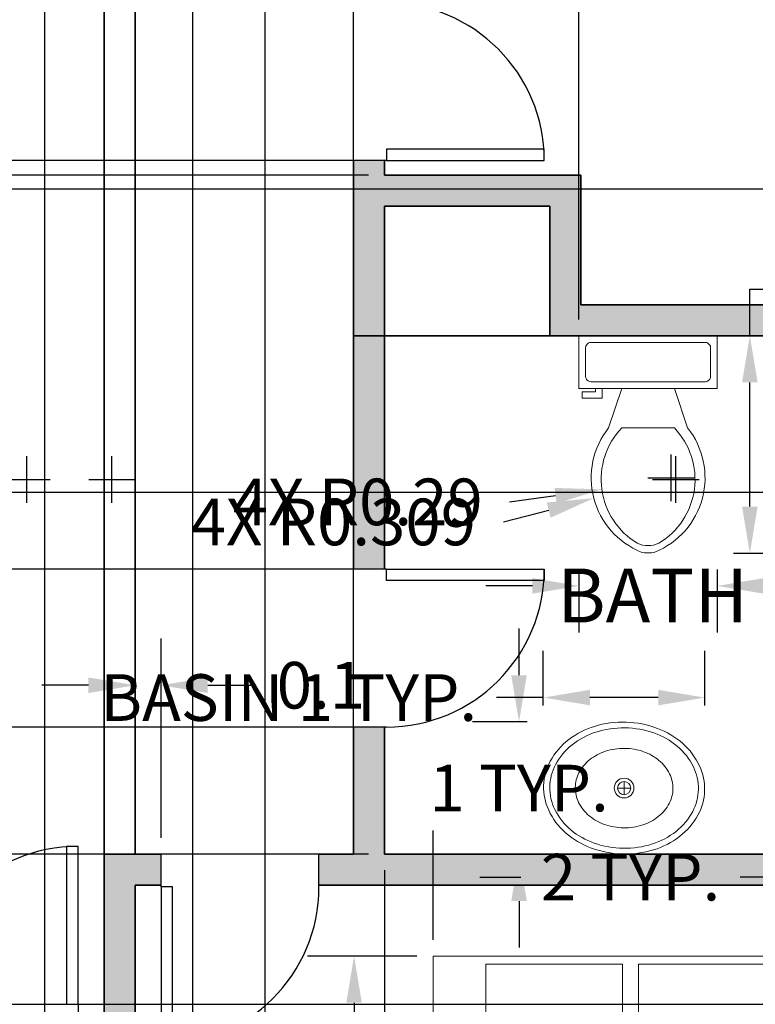
# Model space of a CAD drawing. Units: metres. Extents: x 35.2 to 46.4, y 446.1 to 460.8.
# Tile 3 of 6: x 40.7 to 43.5, y 449.7 to 453.5. Entities that reach past the tile are written whole.
import ezdxf

# ---------------------------------------------------------------- set-up
doc = ezdxf.new("R2010")
doc.units = ezdxf.units.M
for name, color, linetype, lineweight in [('A-ANNO-DIMS', 2, 'Continuous', 18), ('A-AREA-IDEN', 7, 'Continuous', 18), ('A-DOOR', 3, 'Continuous', 25), ('A-WALL', 7, 'Continuous', 35), ('A-WALL-PATT', 252, 'Continuous', 13), ('FURNITURE', 53, 'Continuous', 18), ('SANITARY', 151, 'Continuous', 18)]:
    doc.layers.add(name, color=color, linetype=linetype, lineweight=lineweight)
doc.styles.get("Standard").update_dxf_attribs({"font": 'calibri.ttf'})
doc.dimstyles.get("Standard").update_dxf_attribs({"dimtxt": 0.18, "dimasz": 0.18, "dimexe": 0.18, "dimexo": 0.0625, "dimgap": 0.09, "dimtad": 0, "dimtih": 1, "dimtoh": 1, "dimdec": 4, "dimzin": 0, "dimdsep": 46, "dimtxsty": 'Standard', "dimcen": 0.09, "dimadec": 0, "dimazin": 0, "dimtfac": 1, "dimtdec": 4, "dimtofl": 0, "dimtmove": 0, "dimatfit": 3, "dimfxl": 1, "dimtolj": 1, "dimtzin": 0, "dimarcsym": 0})

# ---------------------------------------------------------------- blocks, each defined once
blk = doc.blocks.new('*U3')
for p, q in [((0, 0), (0, 5)), ((24, 0), (24, 5))]:
    blk.add_line(p, q)
blk.add_lwpolyline([(0, 0), (0, -24), (1.75, -24), (1.75, 0)], close=True)
blk.add_arc((0, 0), 24, 270, 0)
blk = doc.blocks.new('*U4')
for p, q in [((-24, 0), (-24, -5)), ((0, 0), (0, -5))]:
    blk.add_line(p, q)
blk.add_lwpolyline([(0, 0), (0, 24), (-1.75, 24), (-1.75, 0)], close=True)
blk.add_arc((0, 0), 24, 90, 180)
blk = doc.blocks.new('Toilet - top')
for p, q in [((9.5, -6), (9.5, -2)), ((-10, -8.5), (-8, -8.5)), ((-10, -9.5), (-10, -8.5)), ((-8, -8.5), (-8, -8)), ((-7, -8), (-7, -9.5)), ((-4, -8), (-6, -14)), ((4, -8), (6, -14)), ((-7, -9.5), (-10, -9.5)), ((4, -14), (-4, -14))]:
    blk.add_line(p, q)
blk.add_lwpolyline([(10.5, -8), (10.5, 0), (-10.5, 0), (-10.5, -8)], close=True)
for points in [[(8.5, -1), (-8.5, -1)], [(-9.5, -2), (-9.5, -6)], [(-8.5, -7), (8.5, -7)]]:
    blk.add_lwpolyline(points)
for centre, radius, start, end in [((-8.62, -1.88), 0.884, 81.8699, 188.1301), ((8.62, -1.88), 0.884, 351.8699, 98.1301), ((-8.62, -6.12), 0.884, 171.8699, 278.1301), ((8.62, -6.12), 0.884, 261.8699, 8.1301), ((3.52, -21.58), 12.17, 141.4691, 247.9714), ((4.2, -21.82), 11.33, 136.3677, 238.9468), ((-3.52, -21.58), 12.17, 292.0284, 38.5307), ((-4.2, -21.82), 11.33, 301.053, 43.6321), ((0, -27.88), 4, 245.7318, 294.2682), ((0, -29), 4, 254.8605, 285.1395)]:
    blk.add_arc(centre, radius, start, end)
blk = doc.blocks.new('Sink - Oval top')
for p, q in [((-1, 0), (1, 0)), ((0, 1), (0, -1))]:
    blk.add_line(p, q)
for points in [[(-12.23, 0.39, 0.117634), (-11.46, -3.36, 0.104469), (-8.88, -6.8, 0.090016), (-5.08, -9.07, 0.08192), (-0.32, -10.02, 0.08192), (4.49, -9.38, 0.090016), (8.42, -7.36, 0.104469), (11.22, -4.09, 0.117634), (12.23, -0.39, 0.117634), (11.46, 3.36, 0.104469), (8.88, 6.8, 0.090016), (5.08, 9.07, 0.08192), (0.32, 10.02, 0.08192), (-4.49, 9.38, 0.090016), (-8.42, 7.36, 0.104469), (-11.22, 4.09, 0.117634)], [(-11.29, 0.16, 0.118622), (-10.52, -3.25, 0.104678), (-8.07, -6.36, 0.089562), (-4.54, -8.37, 0.081185), (-0.13, -9.15, 0.081185), (4.3, -8.49, 0.089562), (7.89, -6.58, 0.104678), (10.42, -3.55, 0.118622), (11.29, -0.16, 0.118622), (10.52, 3.25, 0.104678), (8.07, 6.36, 0.089562), (4.54, 8.37, 0.081185), (0.13, 9.15, 0.081185), (-4.3, 8.49, 0.089562), (-7.89, 6.58, 0.104678), (-10.42, 3.55, 0.118622)], [(-7.42, 0.08, 0.118283), (-6.91, -2.17, 0.104607), (-5.29, -4.21, 0.089718), (-2.97, -5.53, 0.081436), (-0.07, -6.04, 0.081436), (2.84, -5.59, 0.089718), (5.2, -4.33, 0.104607), (6.86, -2.32, 0.118283), (7.42, -0.08, 0.118283), (6.91, 2.17, 0.104607), (5.29, 4.21, 0.089718), (2.97, 5.53, 0.081436), (0.07, 6.04, 0.081436), (-2.84, 5.59, 0.089718), (-5.2, 4.33, 0.104607), (-6.86, 2.32, 0.118283)]]:
    blk.add_lwpolyline(points, format="xyb", close=True)
for radius in [1.5, 1]:
    blk.add_circle((0, 0), radius)
blk = doc.blocks.new('*U128')
for p, q in [((-24, 0), (-24, 5)), ((0, 0), (0, 5))]:
    blk.add_line(p, q)
blk.add_lwpolyline([(0, 0), (0, -24), (-1.75, -24), (-1.75, 0)], close=True)
blk.add_arc((0, 0), 24, 180, 270)
blk = doc.blocks.new('Bed - Queen')
for p, q in [((0, -80.00003), (0, 0)), ((0, 0), (59.99999, 0)), ((59.99999, 0), (59.99999, -80.00003)), ((7.99999, -1.2), (28.79998, -1.2)), ((7.99999, -14.4), (7.99999, -1.2)), ((28.79998, -1.2), (28.79998, -14.4)), ((31.19999, -1.2), (51.99999, -1.2)), ((31.19999, -14.4), (31.19999, -1.2)), ((51.99999, -1.2), (51.99999, -16.4)), ((0, -14.4), (44.8, -14.4)), ((59.99999, -29.6), (44.8, -14.4)), ((44.8, -14.4), (44.8, -29.6)), ((51.99999, -16.4), (46.79936, -16.4)), ((44.8, -16.8), (0, -16.8)), ((44.8, -29.6), (59.99999, -29.6)), ((59.99999, -80.00003), (0, -80.00003))]:
    blk.add_line(p, q)
blk = doc.blocks.new('*D131')
at = {"layer": 'A-ANNO-DIMS', "color": 0, "lineweight": -2, "transparency": 16777216}
for p, q in [((42.244, 449.8606), (41.8217, 449.8606)), ((42.0017, 449.6806), (42.0017, 449.0387)), ((42.0017, 448.0086), (42.0017, 448.6505)), ((42.244, 447.8286), (41.8217, 447.8286))]:
    blk.add_line(p, q, dxfattribs=at)
at = {"layer": 'A-ANNO-DIMS', "color": 0, "transparency": 16777216}
for points in [[(41.9717, 449.6806), (42.0317, 449.6806), (42.0017, 449.8606)], [(41.9717, 448.0086), (42.0317, 448.0086), (42.0017, 447.8286)]]:
    blk.add_solid(points, dxfattribs=at)
at = {"layer": 'Defpoints', "color": 0, "transparency": 16777216}
for p in [(42.0017, 449.8606), (42.3065, 449.8606), (42.3065, 447.8286)]:
    blk.add_point(p, dxfattribs=at)
at = {"layer": 'A-ANNO-DIMS', "color": 0, "transparency": 16777216, "insert": (42.0017, 448.8446), "char_height": 0.18, "attachment_point": 5}
blk.add_mtext('\\A1;QUEEN BED 2 TYP.', dxfattribs=at)
blk = doc.blocks.new('*D132')
at = {"layer": 'A-ANNO-DIMS', "color": 0, "lineweight": -2, "transparency": 16777216}
for p, q in [((42.3065, 449.9231), (42.3065, 450.3454)), ((43.8305, 449.9231), (43.8305, 450.3454)), ((42.4865, 450.1654), (42.6457, 450.1654)), ((43.6505, 450.1654), (43.4913, 450.1654))]:
    blk.add_line(p, q, dxfattribs=at)
at = {"layer": 'A-ANNO-DIMS', "color": 0, "transparency": 16777216}
for points in [[(42.4865, 450.1954), (42.4865, 450.1354), (42.3065, 450.1654)], [(43.6505, 450.1954), (43.6505, 450.1354), (43.8305, 450.1654)]]:
    blk.add_solid(points, dxfattribs=at)
at = {"layer": 'Defpoints', "color": 0, "transparency": 16777216}
for p in [(43.8305, 450.1654), (42.3065, 449.8606), (43.8305, 449.8606)]:
    blk.add_point(p, dxfattribs=at)
at = {"layer": 'A-ANNO-DIMS', "color": 0, "transparency": 16777216, "insert": (43.0685, 450.1654), "char_height": 0.18, "attachment_point": 5}
blk.add_mtext('\\A1;2 TYP.', dxfattribs=at)
blk = doc.blocks.new('*D135')
at = {"layer": 'A-ANNO-DIMS', "color": 0, "lineweight": -2, "transparency": 16777216}
for p, q in [((43.5288, 452.2548), (43.5288, 452.4348)), ((43.5288, 452.4348), (43.7088, 452.4348)), ((43.4654, 452.2548), (43.7088, 452.2548)), ((43.5288, 451.5954), (43.5288, 452.0748)), ((43.4654, 451.4154), (43.7088, 451.4154))]:
    blk.add_line(p, q, dxfattribs=at)
at = {"layer": 'A-ANNO-DIMS', "color": 0, "transparency": 16777216}
for points in [[(43.4988, 452.0748), (43.5588, 452.0748), (43.5288, 452.2548)], [(43.4988, 451.5954), (43.5588, 451.5954), (43.5288, 451.4154)]]:
    blk.add_solid(points, dxfattribs=at)
at = {"layer": 'Defpoints', "color": 0, "transparency": 16777216}
for p in [(43.4029, 452.2548), (43.5288, 452.2548), (43.4029, 451.4154)]:
    blk.add_point(p, dxfattribs=at)
at = {"layer": 'A-ANNO-DIMS', "color": 0, "transparency": 16777216, "insert": (44.3691, 452.4348), "char_height": 0.18, "attachment_point": 5}
blk.add_mtext('\\A1;WC 1 TYP.', dxfattribs=at)
blk = doc.blocks.new('*D136')
at = {"layer": 'A-ANNO-DIMS', "color": 0, "lineweight": -2, "transparency": 16777216}
for p, q in [((42.8695, 451.3529), (42.8695, 451.1095)), ((43.4029, 451.3529), (43.4029, 451.1095)), ((42.6895, 451.2895), (42.5095, 451.2895)), ((43.5829, 451.2895), (43.7629, 451.2895))]:
    blk.add_line(p, q, dxfattribs=at)
at = {"layer": 'A-ANNO-DIMS', "color": 0, "transparency": 16777216}
for points in [[(42.6895, 451.3195), (42.6895, 451.2595), (42.8695, 451.2895)], [(43.5829, 451.3195), (43.5829, 451.2595), (43.4029, 451.2895)]]:
    blk.add_solid(points, dxfattribs=at)
at = {"layer": 'Defpoints', "color": 0, "transparency": 16777216}
for p in [(42.8695, 451.4154), (43.4029, 451.4154), (43.4029, 451.2895)]:
    blk.add_point(p, dxfattribs=at)
at = {"layer": 'A-ANNO-DIMS', "color": 0, "transparency": 16777216, "insert": (44.1815, 451.2895), "char_height": 0.18, "attachment_point": 5}
blk.add_mtext('\\A1;1 TYP.', dxfattribs=at)
blk = doc.blocks.new('*D137')
at = {"layer": 'A-ANNO-DIMS', "color": 0, "lineweight": -2, "transparency": 16777216}
for p, q in [((42.7318, 450.8274), (42.7318, 451.0385)), ((43.3554, 450.8274), (43.3554, 451.0385)), ((42.7318, 450.8585), (42.5518, 450.8585)), ((43.1754, 450.8585), (42.9118, 450.8585))]:
    blk.add_line(p, q, dxfattribs=at)
at = {"layer": 'A-ANNO-DIMS', "color": 0, "transparency": 16777216}
for points in [[(42.9118, 450.8885), (42.9118, 450.8285), (42.7318, 450.8585)], [(43.1754, 450.8885), (43.1754, 450.8285), (43.3554, 450.8585)]]:
    blk.add_solid(points, dxfattribs=at)
at = {"layer": 'Defpoints', "color": 0, "transparency": 16777216}
for p in [(42.7318, 450.8585), (42.7318, 450.7649), (43.3554, 450.7649)]:
    blk.add_point(p, dxfattribs=at)
at = {"layer": 'A-ANNO-DIMS', "color": 0, "transparency": 16777216, "insert": (41.7494, 450.8585), "char_height": 0.18, "attachment_point": 5}
blk.add_mtext('\\A1;BASIN 1 TYP.', dxfattribs=at)
blk = doc.blocks.new('*D138')
at = {"layer": 'A-ANNO-DIMS', "color": 0, "lineweight": -2, "transparency": 16777216}
for p, q in [((42.6382, 450.9449), (42.6382, 451.1249)), ((42.6693, 450.7649), (42.4582, 450.7649)), ((42.6693, 450.2534), (42.4582, 450.2534)), ((42.6382, 450.0734), (42.6382, 449.8934))]:
    blk.add_line(p, q, dxfattribs=at)
at = {"layer": 'A-ANNO-DIMS', "color": 0, "transparency": 16777216}
for points in [[(42.6082, 450.9449), (42.6682, 450.9449), (42.6382, 450.7649)], [(42.6082, 450.0734), (42.6682, 450.0734), (42.6382, 450.2534)]]:
    blk.add_solid(points, dxfattribs=at)
at = {"layer": 'Defpoints', "color": 0, "transparency": 16777216}
for p in [(42.7318, 450.7649), (42.6382, 450.2534), (42.7318, 450.2534)]:
    blk.add_point(p, dxfattribs=at)
at = {"layer": 'A-ANNO-DIMS', "color": 0, "transparency": 16777216, "insert": (42.6382, 450.5092), "char_height": 0.18, "attachment_point": 5}
blk.add_mtext('\\A1;1 TYP.', dxfattribs=at)
blk = doc.blocks.new('*D155')
at = {"layer": 'A-ANNO-DIMS', "color": 0, "lineweight": -2, "transparency": 16777216}
for p, q in [((37.8991, 451.6506), (45.8178, 451.6506)), ((45.6378, 451.4706), (45.6378, 450.8449)), ((45.6378, 449.8548), (45.6378, 450.4805)), ((37.8991, 449.6748), (45.8178, 449.6748))]:
    blk.add_line(p, q, dxfattribs=at)
at = {"layer": 'A-ANNO-DIMS', "color": 0, "transparency": 16777216}
for points in [[(45.6078, 451.4706), (45.6678, 451.4706), (45.6378, 451.6506)], [(45.6078, 449.8548), (45.6678, 449.8548), (45.6378, 449.6748)]]:
    blk.add_solid(points, dxfattribs=at)
at = {"layer": 'Defpoints', "color": 0, "transparency": 16777216}
for p in [(37.8366, 451.6506), (45.6378, 451.6506), (37.8366, 449.6748)]:
    blk.add_point(p, dxfattribs=at)
at = {"layer": 'A-ANNO-DIMS', "color": 0, "transparency": 16777216, "insert": (45.6378, 450.6627), "char_height": 0.18, "attachment_point": 5}
blk.add_mtext('\\A1;1.976', dxfattribs=at)
blk = doc.blocks.new('*D156')
at = {"layer": 'A-ANNO-DIMS', "color": 0, "lineweight": -2, "transparency": 16777216}
for p, q in [((37.8991, 455.122), (45.8178, 455.122)), ((45.6378, 454.942), (45.6378, 454.1543)), ((45.6378, 453.0022), (45.6378, 453.7898)), ((37.8991, 452.8222), (45.8178, 452.8222))]:
    blk.add_line(p, q, dxfattribs=at)
at = {"layer": 'A-ANNO-DIMS', "color": 0, "transparency": 16777216}
for points in [[(45.6078, 454.942), (45.6678, 454.942), (45.6378, 455.122)], [(45.6078, 453.0022), (45.6678, 453.0022), (45.6378, 452.8222)]]:
    blk.add_solid(points, dxfattribs=at)
at = {"layer": 'Defpoints', "color": 0, "transparency": 16777216}
for p in [(37.8366, 455.122), (45.6378, 455.122), (37.8366, 452.8222)]:
    blk.add_point(p, dxfattribs=at)
at = {"layer": 'A-ANNO-DIMS', "color": 0, "transparency": 16777216, "insert": (45.6378, 453.9721), "char_height": 0.18, "attachment_point": 5}
blk.add_mtext('\\A1;2.3', dxfattribs=at)
blk = doc.blocks.new('*D167')
at = {"layer": 'A-ANNO-DIMS', "color": 0, "lineweight": -2, "transparency": 16777216}
for p, q in [((37.8366, 459.6323), (37.8366, 446.0736)), ((40.8069, 459.6323), (40.8069, 446.0736)), ((38.0166, 446.2536), (38.9948, 446.2536)), ((40.6269, 446.2536), (39.6486, 446.2536))]:
    blk.add_line(p, q, dxfattribs=at)
at = {"layer": 'A-ANNO-DIMS', "color": 0, "transparency": 16777216}
for points in [[(38.0166, 446.2836), (38.0166, 446.2236), (37.8366, 446.2536)], [(40.6269, 446.2836), (40.6269, 446.2236), (40.8069, 446.2536)]]:
    blk.add_solid(points, dxfattribs=at)
at = {"layer": 'Defpoints', "color": 0, "transparency": 16777216}
for p in [(37.8366, 459.6948), (40.8069, 459.6948), (40.8069, 446.2536)]:
    blk.add_point(p, dxfattribs=at)
at = {"layer": 'A-ANNO-DIMS', "color": 0, "transparency": 16777216, "insert": (39.3217, 446.2536), "char_height": 0.18, "attachment_point": 5}
blk.add_mtext('\\A1;2.97', dxfattribs=at)
blk = doc.blocks.new('*D168')
at = {"layer": 'A-ANNO-DIMS', "color": 0, "lineweight": -2, "transparency": 16777216}
for p, q in [((40.8069, 459.6323), (40.8069, 446.0736)), ((41.3784, 459.6323), (41.3784, 446.0736)), ((40.9869, 446.2536), (41.1984, 446.2536)), ((41.3784, 446.2536), (41.5584, 446.2536))]:
    blk.add_line(p, q, dxfattribs=at)
at = {"layer": 'A-ANNO-DIMS', "color": 0, "transparency": 16777216}
for points in [[(40.9869, 446.2836), (40.9869, 446.2236), (40.8069, 446.2536)], [(41.1984, 446.2836), (41.1984, 446.2236), (41.3784, 446.2536)]]:
    blk.add_solid(points, dxfattribs=at)
at = {"layer": 'Defpoints', "color": 0, "transparency": 16777216}
for p in [(40.8069, 459.6948), (41.3784, 459.6948), (41.3784, 446.2536)]:
    blk.add_point(p, dxfattribs=at)
at = {"layer": 'A-ANNO-DIMS', "color": 0, "transparency": 16777216, "insert": (41.8883, 446.2536), "char_height": 0.18, "attachment_point": 5}
blk.add_mtext('\\A1;0.57', dxfattribs=at)
blk = doc.blocks.new('*D169')
at = {"layer": 'A-ANNO-DIMS', "color": 0, "lineweight": -2, "transparency": 16777216}
for p, q in [((40.536595, 457.132279), (40.536595, 446.073579)), ((41.656595, 457.132279), (41.656595, 446.073579)), ((40.356595, 446.253579), (40.176595, 446.253579)), ((41.836595, 446.253579), (42.016595, 446.253579))]:
    blk.add_line(p, q, dxfattribs=at)
at = {"layer": 'A-ANNO-DIMS', "color": 0, "transparency": 16777216}
for points in [[(40.356595, 446.283579), (40.356595, 446.223579), (40.536595, 446.253579)], [(41.836595, 446.283579), (41.836595, 446.223579), (41.656595, 446.253579)]]:
    blk.add_solid(points, dxfattribs=at)
at = {"layer": 'Defpoints', "color": 0, "transparency": 16777216}
for p in [(40.536595, 457.194779), (41.656595, 457.194779), (41.656595, 446.253579)]:
    blk.add_point(p, dxfattribs=at)
at = {"layer": 'A-ANNO-DIMS', "color": 0, "transparency": 16777216, "insert": (41.096595, 446.253579), "char_height": 0.18, "attachment_point": 5}
blk.add_mtext('\\A1;1.12', dxfattribs=at)
blk = doc.blocks.new('*D171')
at = {"layer": 'A-ANNO-DIMS', "color": 0, "lineweight": -2, "transparency": 16777216}
for p, q in [((42.1191, 450.1923), (42.1191, 446.0736)), ((44.7566, 450.1923), (44.7566, 446.0736)), ((42.2991, 446.2536), (43.1085, 446.2536)), ((44.5766, 446.2536), (43.7673, 446.2536))]:
    blk.add_line(p, q, dxfattribs=at)
at = {"layer": 'A-ANNO-DIMS', "color": 0, "transparency": 16777216}
for points in [[(42.2991, 446.2836), (42.2991, 446.2236), (42.1191, 446.2536)], [(44.5766, 446.2836), (44.5766, 446.2236), (44.7566, 446.2536)]]:
    blk.add_solid(points, dxfattribs=at)
at = {"layer": 'Defpoints', "color": 0, "transparency": 16777216}
for p in [(42.1191, 450.2548), (44.7566, 450.2548), (44.7566, 446.2536)]:
    blk.add_point(p, dxfattribs=at)
at = {"layer": 'A-ANNO-DIMS', "color": 0, "transparency": 16777216, "insert": (43.4379, 446.2536), "char_height": 0.18, "attachment_point": 5}
blk.add_mtext('\\A1;2.64', dxfattribs=at)
blk = doc.blocks.new('*D180')
at = {"layer": 'A-ANNO-DIMS', "color": 0, "lineweight": -2, "transparency": 16777216}
for p, q in [((36.9554, 450.9246), (36.9554, 451.1046)), ((42.0566, 450.7446), (36.7754, 450.7446)), ((42.0566, 450.2548), (36.7754, 450.2548)), ((36.9554, 450.0748), (36.9554, 449.8948))]:
    blk.add_line(p, q, dxfattribs=at)
at = {"layer": 'A-ANNO-DIMS', "color": 0, "transparency": 16777216}
for points in [[(36.9254, 450.9246), (36.9854, 450.9246), (36.9554, 450.7446)], [(36.9254, 450.0748), (36.9854, 450.0748), (36.9554, 450.2548)]]:
    blk.add_solid(points, dxfattribs=at)
at = {"layer": 'Defpoints', "color": 0, "transparency": 16777216}
for p in [(36.9554, 450.7446), (42.1191, 450.7446), (42.1191, 450.2548)]:
    blk.add_point(p, dxfattribs=at)
at = {"layer": 'A-ANNO-DIMS', "color": 0, "transparency": 16777216, "insert": (36.9554, 450.4997), "char_height": 0.18, "attachment_point": 5}
blk.add_mtext('\\A1;0.49', dxfattribs=at)
blk = doc.blocks.new('*D181')
at = {"layer": 'A-ANNO-DIMS', "color": 0, "lineweight": -2, "transparency": 16777216}
for p, q in [((36.9554, 451.3542), (36.9554, 451.5342)), ((36.9554, 451.5342), (37.1354, 451.5342)), ((42.0566, 451.3542), (36.7754, 451.3542)), ((36.9554, 450.9246), (36.9554, 451.1742)), ((42.0566, 450.7446), (36.7754, 450.7446))]:
    blk.add_line(p, q, dxfattribs=at)
at = {"layer": 'A-ANNO-DIMS', "color": 0, "transparency": 16777216}
for points in [[(36.9254, 451.1742), (36.9854, 451.1742), (36.9554, 451.3542)], [(36.9254, 450.9246), (36.9854, 450.9246), (36.9554, 450.7446)]]:
    blk.add_solid(points, dxfattribs=at)
at = {"layer": 'Defpoints', "color": 0, "transparency": 16777216}
for p in [(36.9554, 451.3542), (42.1191, 451.3542), (42.1191, 450.7446)]:
    blk.add_point(p, dxfattribs=at)
at = {"layer": 'A-ANNO-DIMS', "color": 0, "transparency": 16777216, "insert": (37.4641, 451.5342), "char_height": 0.18, "attachment_point": 5}
blk.add_mtext('\\A1;0.61', dxfattribs=at)
blk = doc.blocks.new('*D182')
at = {"layer": 'A-ANNO-DIMS', "color": 0, "lineweight": -2, "transparency": 16777216}
for p, q in [((41.9991, 452.3173), (41.9991, 460.756)), ((42.8695, 452.3173), (42.8695, 460.756)), ((41.8191, 460.576), (41.6391, 460.576)), ((43.0495, 460.576), (43.2295, 460.576))]:
    blk.add_line(p, q, dxfattribs=at)
at = {"layer": 'A-ANNO-DIMS', "color": 0, "transparency": 16777216}
for points in [[(41.8191, 460.606), (41.8191, 460.546), (41.9991, 460.576)], [(43.0495, 460.606), (43.0495, 460.546), (42.8695, 460.576)]]:
    blk.add_solid(points, dxfattribs=at)
at = {"layer": 'Defpoints', "color": 0, "transparency": 16777216}
for p in [(42.8695, 460.576), (41.9991, 452.2548), (42.8695, 452.2548)]:
    blk.add_point(p, dxfattribs=at)
at = {"layer": 'A-ANNO-DIMS', "color": 0, "transparency": 16777216, "insert": (42.4343, 460.576), "char_height": 0.18, "attachment_point": 5}
blk.add_mtext('\\A1;0.87', dxfattribs=at)
blk = doc.blocks.new('*D183')
at = {"layer": 'A-ANNO-DIMS', "color": 0, "lineweight": -2, "transparency": 16777216}
for p, q in [((41.1566, 450.3173), (41.1566, 460.756)), ((41.9991, 450.3173), (41.9991, 460.756)), ((40.9766, 460.576), (40.7966, 460.576)), ((42.1791, 460.576), (42.3591, 460.576))]:
    blk.add_line(p, q, dxfattribs=at)
at = {"layer": 'A-ANNO-DIMS', "color": 0, "transparency": 16777216}
for points in [[(40.9766, 460.606), (40.9766, 460.546), (41.1566, 460.576)], [(42.1791, 460.606), (42.1791, 460.546), (41.9991, 460.576)]]:
    blk.add_solid(points, dxfattribs=at)
at = {"layer": 'Defpoints', "color": 0, "transparency": 16777216}
for p in [(41.9991, 460.576), (41.1566, 450.2548), (41.9991, 450.2548)]:
    blk.add_point(p, dxfattribs=at)
at = {"layer": 'A-ANNO-DIMS', "color": 0, "transparency": 16777216, "insert": (41.5779, 460.576), "char_height": 0.18, "attachment_point": 5}
blk.add_mtext('\\A1;0.84', dxfattribs=at)
blk = doc.blocks.new('*D185')
at = {"layer": 'A-ANNO-DIMS', "color": 0, "lineweight": -2, "transparency": 16777216}
for p, q in [((41.1566, 450.3173), (41.1566, 451.086)), ((41.2566, 450.3173), (41.2566, 451.086)), ((40.9766, 450.906), (40.7966, 450.906)), ((41.4366, 450.906), (41.6166, 450.906))]:
    blk.add_line(p, q, dxfattribs=at)
at = {"layer": 'A-ANNO-DIMS', "color": 0, "transparency": 16777216}
for points in [[(40.9766, 450.936), (40.9766, 450.876), (41.1566, 450.906)], [(41.4366, 450.936), (41.4366, 450.876), (41.2566, 450.906)]]:
    blk.add_solid(points, dxfattribs=at)
at = {"layer": 'Defpoints', "color": 0, "transparency": 16777216}
for p in [(41.2566, 450.906), (41.1566, 450.2548), (41.2566, 450.2548)]:
    blk.add_point(p, dxfattribs=at)
at = {"layer": 'A-ANNO-DIMS', "color": 0, "transparency": 16777216, "insert": (41.8734, 450.906), "char_height": 0.18, "attachment_point": 5}
blk.add_mtext('\\A1;0.1', dxfattribs=at)
blk = doc.blocks.new('*D186')
at = {"layer": 'A-ANNO-DIMS', "color": 0, "lineweight": -2, "transparency": 16777216}
for p, q in [((36.9554, 453.1107), (36.9554, 453.2907)), ((36.9554, 453.2907), (37.1354, 453.2907)), ((42.0566, 452.9307), (36.7754, 452.9307)), ((42.0566, 452.8748), (36.7754, 452.8748)), ((36.9554, 452.6948), (36.9554, 452.5148))]:
    blk.add_line(p, q, dxfattribs=at)
at = {"layer": 'A-ANNO-DIMS', "color": 0, "transparency": 16777216}
for points in [[(36.9254, 453.1107), (36.9854, 453.1107), (36.9554, 452.9307)], [(36.9254, 452.6948), (36.9854, 452.6948), (36.9554, 452.8748)]]:
    blk.add_solid(points, dxfattribs=at)
at = {"layer": 'Defpoints', "color": 0, "transparency": 16777216}
for p in [(36.9554, 452.9307), (42.1191, 452.9307), (42.1191, 452.8748)]:
    blk.add_point(p, dxfattribs=at)
at = {"layer": 'A-ANNO-DIMS', "color": 0, "transparency": 16777216, "insert": (37.538, 453.2907), "char_height": 0.18, "attachment_point": 5}
blk.add_mtext('\\A1;0.056', dxfattribs=at)
blk = doc.blocks.new('*D187')
at = {"layer": 'A-ANNO-DIMS', "color": 0, "lineweight": -2, "transparency": 16777216}
for p, q in [((41.0674, 451.6101), (41.0674, 451.7901)), ((36.142, 451.6999), (37.809, 451.7)), ((40.9774, 451.7001), (41.1574, 451.7001))]:
    blk.add_line(p, q, dxfattribs=at)
at = {"layer": 'A-ANNO-DIMS', "color": 0, "transparency": 16777216}
blk.add_solid([(37.809, 451.73), (37.809, 451.67), (37.989, 451.7)], dxfattribs=at)
at = {"layer": 'Defpoints', "color": 0, "transparency": 16777216}
for p in [(37.989, 451.7), (41.0674, 451.7001)]:
    blk.add_point(p, dxfattribs=at)
at = {"layer": 'A-ANNO-DIMS', "color": 0, "transparency": 16777216, "insert": (35.7413, 451.6999), "char_height": 0.18, "attachment_point": 5}
blk.add_mtext('\\A1;R3.08', dxfattribs=at)
blk = doc.blocks.new('*D188')
at = {"layer": 'A-ANNO-DIMS', "color": 0, "lineweight": -2, "transparency": 16777216}
for p, q in [((40.7385, 451.6101), (40.7385, 451.7901)), ((36.0954, 451.6999), (37.6566, 451.7)), ((40.6485, 451.7001), (40.8285, 451.7001))]:
    blk.add_line(p, q, dxfattribs=at)
at = {"layer": 'A-ANNO-DIMS', "color": 0, "transparency": 16777216}
blk.add_solid([(37.6566, 451.73), (37.6566, 451.67), (37.8366, 451.7)], dxfattribs=at)
at = {"layer": 'Defpoints', "color": 0, "transparency": 16777216}
for p in [(37.8366, 451.7), (40.7385, 451.7001)]:
    blk.add_point(p, dxfattribs=at)
at = {"layer": 'A-ANNO-DIMS', "color": 0, "transparency": 16777216, "insert": (35.625, 451.6999), "char_height": 0.18, "attachment_point": 5}
blk.add_mtext('\\A1;R2.902', dxfattribs=at)
blk = doc.blocks.new('*D190')
at = {"layer": 'A-ANNO-DIMS', "color": 0, "lineweight": -2, "transparency": 16777216}
for p, q in [((43.2256, 451.6166), (43.2256, 451.7966)), ((43.1356, 451.7066), (43.3156, 451.7066)), ((42.5786, 451.5362), (42.7526, 451.5821))]:
    blk.add_line(p, q, dxfattribs=at)
at = {"layer": 'A-ANNO-DIMS', "color": 0, "transparency": 16777216}
blk.add_solid([(42.745, 451.6111), (42.7603, 451.5531), (42.9267, 451.6279)], dxfattribs=at)
at = {"layer": 'Defpoints', "color": 0, "transparency": 16777216}
for p in [(43.2256, 451.7066), (42.9267, 451.6279)]:
    blk.add_point(p, dxfattribs=at)
at = {"layer": 'A-ANNO-DIMS', "color": 0, "transparency": 16777216, "insert": (41.9214, 451.5362), "char_height": 0.18, "attachment_point": 5}
blk.add_mtext('\\A1;4X R0.309', dxfattribs=at)
blk = doc.blocks.new('*D191')
at = {"layer": 'A-ANNO-DIMS', "color": 0, "lineweight": -2, "transparency": 16777216}
for p, q in [((43.2429, 451.6106), (43.2429, 451.7906)), ((43.1529, 451.7006), (43.3329, 451.7006)), ((42.601, 451.6136), (42.7794, 451.6378))]:
    blk.add_line(p, q, dxfattribs=at)
at = {"layer": 'A-ANNO-DIMS', "color": 0, "transparency": 16777216}
blk.add_solid([(42.7753, 451.6675), (42.7834, 451.6081), (42.9577, 451.662)], dxfattribs=at)
at = {"layer": 'Defpoints', "color": 0, "transparency": 16777216}
for p in [(43.2429, 451.7006), (42.9577, 451.662)]:
    blk.add_point(p, dxfattribs=at)
at = {"layer": 'A-ANNO-DIMS', "color": 0, "transparency": 16777216, "insert": (42.0156, 451.6136), "char_height": 0.18, "attachment_point": 5}
blk.add_mtext('\\A1;4X R0.29', dxfattribs=at)

msp = doc.modelspace()

# ---------------------------------------------------------------- hatches: boundary and pattern name
at = {"layer": 'A-WALL-PATT'}
h = msp.add_hatch(color=256, dxfattribs=at)
h.dxf.hatch_style = 1
h.paths.add_polyline_path([(37.8366, 451.6506), (37.6066, 451.6506), (37.6066, 449.5548), (40.327, 449.5548), (40.327, 449.6748), (37.8366, 449.6748)])
h.paths.add_polyline_path([(37.8366, 455.122), (37.6066, 455.122), (37.6066, 452.8222), (37.8366, 452.8222)])
h.paths.add_polyline_path([(37.8366, 457.0257), (37.8366, 457.0747), (37.8341, 457.0771), (37.8366, 457.0796), (37.8366, 457.1285), (37.8341, 457.131), (37.8366, 457.1335), (37.8366, 457.1824), (37.8341, 457.1849), (37.8366, 457.1874), (37.8366, 457.2363), (37.8341, 457.2388), (37.8366, 457.2412), (37.8366, 457.2902), (37.8341, 457.2927), (37.8366, 457.2951), (37.8366, 457.3441), (37.8341, 457.3465), (37.8366, 457.349), (37.8366, 457.398), (37.8341, 457.4004), (37.8366, 457.4029), (37.8366, 457.4518), (37.8341, 457.4543), (37.8366, 457.4568), (37.8366, 457.5057), (37.8341, 457.5082), (37.8366, 457.5107), (37.8366, 457.5596), (37.8341, 457.5621), (37.8366, 457.5645), (37.8366, 457.6135), (37.8341, 457.6159), (37.8366, 457.6184), (37.8366, 457.6674), (37.8341, 457.6698), (37.8366, 457.6723), (37.8366, 457.7212), (37.8341, 457.7237), (37.8366, 457.7262), (37.8366, 457.7751), (37.8341, 457.7776), (37.8366, 457.7801), (37.8366, 457.829), (37.8341, 457.8315), (37.8366, 457.8339), (37.8366, 457.8829), (37.8341, 457.8854), (37.8366, 457.8878), (37.8366, 457.9368), (37.8341, 457.9392), (37.8366, 457.9417), (37.8366, 457.9906), (37.8341, 457.9931), (37.8366, 457.9956), (37.8366, 458.0445), (37.8341, 458.047), (37.8366, 458.0495), (37.8366, 458.0984), (37.8341, 458.1009), (37.8366, 458.1033), (37.8366, 458.1523), (37.8272, 458.1617), (37.6066, 458.1617), (37.6066, 456.2935), (37.8366, 456.2935), (37.8366, 457.0208), (37.8341, 457.0232)], flags=17)
h.paths.add_polyline_path([(40.8069, 459.9248), (37.6066, 459.9248), (37.6066, 459.3333), (37.8273, 459.3333), (37.8366, 459.3426), (37.8366, 459.3916), (37.8341, 459.394), (37.8366, 459.3965), (37.8366, 459.4455), (37.8341, 459.4479), (37.8366, 459.4504), (37.8366, 459.4993), (37.8341, 459.5018), (37.8366, 459.5043), (37.8366, 459.5532), (37.8341, 459.5557), (37.8366, 459.5582), (37.8366, 459.6071), (37.8341, 459.6096), (37.8366, 459.612), (37.8366, 459.661), (37.8341, 459.6634), (37.8366, 459.6659), (37.8366, 459.6948), (40.4166, 459.6948), (40.4166, 457.0748), (41.0366, 457.0748), (41.0366, 455.1347), (41.1566, 455.1347), (41.1566, 455.9748), (41.2566, 455.9748), (41.2566, 456.0948), (41.1566, 456.0948), (41.1566, 457.0748), (41.7766, 457.0748), (41.7766, 459.6948), (44.7566, 459.6948), (44.7566, 458.3327), (44.9866, 458.3327), (44.9866, 459.9248), (41.3784, 459.9248), (41.3784, 459.6948), (41.6566, 459.6948), (41.6566, 457.1948), (40.5366, 457.1948), (40.5366, 459.6948), (40.8069, 459.6948)])
h.paths.add_polyline_path([(42.1191, 452.2548), (41.9991, 452.2548), (41.9991, 451.3542), (42.1191, 451.3542)])
h = msp.add_hatch(color=256, dxfattribs=at)
h.dxf.hatch_style = 1
h.paths.add_polyline_path([(44.9866, 457.1611), (44.7566, 457.1611), (44.7566, 454.5208), (44.9866, 454.5208)])
h.paths.add_polyline_path([(44.9866, 453.3493), (44.7566, 453.3493), (44.7566, 452.3748), (42.8766, 452.3748), (42.8766, 452.8748), (42.1191, 452.8748), (42.1191, 452.9307), (41.9991, 452.9307), (41.9991, 452.2548), (42.1191, 452.2548), (42.1191, 452.7548), (42.7566, 452.7548), (42.7566, 452.2548), (44.7566, 452.2548), (44.7566, 451.6519), (44.9866, 451.6519)])
h.paths.add_polyline_path([(44.9866, 451.0803), (44.7566, 451.0803), (44.7566, 450.2548), (43.6593, 450.2548), (43.0598, 450.2548, -0.016107), (43.0354, 450.2548), (42.1191, 450.2548), (42.1191, 450.7446), (41.9991, 450.7446), (41.9991, 450.2548), (41.8662, 450.2548), (41.8662, 450.1348), (44.7566, 450.1348), (44.7566, 448.5414), (44.9866, 448.5414)])
h.paths.add_polyline_path([(44.9866, 447.3698), (44.7566, 447.3698), (44.7566, 447.1348), (41.1566, 447.1348), (41.1566, 450.1348), (41.2566, 450.1348), (41.2566, 450.2548), (41.0366, 450.2548), (41.0366, 446.9048), (44.9866, 446.9048)])

# ---------------------------------------------------------------- linework, layer by layer
at = {"layer": 'A-WALL', "transparency": 33554534}
for p, q in [((41.1566, 454.3347), (41.1566, 450.2548)), ((41.0366, 450.2548), (41.0366, 454.2147))]:
    msp.add_line(p, q, dxfattribs=at)
at = {"layer": 'A-WALL'}
for p, q in [((41.9991, 452.9307), (41.9991, 451.3542)), ((42.1191, 452.9307), (42.1191, 452.8748)), ((42.1191, 452.8748), (42.8766, 452.8748)), ((42.8766, 452.8748), (42.8766, 452.3748)), ((42.1191, 452.7548), (42.7566, 452.7548)), ((42.1191, 452.7548), (42.1191, 451.3542)), ((42.7566, 452.7548), (42.7566, 452.2548)), ((42.8766, 452.3748), (44.7566, 452.3748)), ((41.9991, 452.2548), (44.7566, 452.2548)), ((41.9991, 450.7446), (41.9991, 450.2548)), ((42.1191, 450.7446), (42.1191, 450.2548)), ((41.0366, 450.2548), (41.0366, 446.9048)), ((41.0366, 450.2548), (41.2566, 450.2548)), ((41.8662, 450.2548), (41.9991, 450.2548)), ((42.1191, 450.2548), (44.7566, 450.2548)), ((41.1566, 450.1348), (41.2566, 450.1348)), ((41.1566, 450.1348), (41.1566, 447.1348)), ((41.8662, 450.1348), (44.7566, 450.1348))]:
    msp.add_line(p, q, dxfattribs=at)

# ---------------------------------------------------------------- block references
at = {"layer": 'A-DOOR', "xscale": 0.0254, "yscale": 0.0254, "zscale": 0.0254, "rotation": 90}
for name, p in [('*U3', (42.1261, 452.9307)), ('*U128', (42.1261, 451.3542))]:
    msp.add_blockref(name, p, dxfattribs=at)
at = {"layer": 'A-DOOR', "xscale": 0.0254, "yscale": 0.0254, "zscale": 0.0254}
for name, p in [('*U4', (40.9366, 449.6748)), ('*U3', (41.2566, 450.1278))]:
    msp.add_blockref(name, p, dxfattribs=at)
at = {"layer": 'FURNITURE', "transparency": 33554521, "xscale": 0.0254, "yscale": 0.0254, "zscale": 0.0254}
msp.add_blockref('Bed - Queen', (42.3065, 449.8606), dxfattribs=at)
at = {"layer": 'SANITARY', "transparency": 33554521, "xscale": 0.0254, "yscale": 0.0254, "zscale": 0.0254}
msp.add_blockref('Toilet - top', (43.1362, 452.2548), dxfattribs=at)
at = {"layer": 'SANITARY', "transparency": 33554521, "xscale": 0.0254, "yscale": 0.0254, "zscale": 0.0254, "rotation": 180}
msp.add_blockref('Sink - Oval top', (43.0436, 450.5092), dxfattribs=at)

# ---------------------------------------------------------------- texts
at = {"layer": 'A-AREA-IDEN'}
msp.add_text('BATH', height=0.20807, dxfattribs=at).set_placement((42.7858, 451.1483))

# ---------------------------------------------------------------- dimensions: what is measured, and where the dimension line sits
at = {"layer": 'A-ANNO-DIMS'}
for base, p1, p2, override, picture, middle in [((41.9991, 460.576), (41.1566, 450.2548), (41.9991, 450.2548), {"dimdec": 2, "dimlfac": 1, "dimrnd": 0, "dimzin": 0, "dimdsep": 46, "dimlunit": 2}, '*D183', (41.5779, 460.576)), ((42.8695, 460.576), (41.9991, 452.2548), (42.8695, 452.2548), {"dimdec": 2, "dimlfac": 1, "dimrnd": 0, "dimzin": 0, "dimdsep": 46, "dimlunit": 2}, '*D182', (42.4343, 460.576)), ((40.8069, 446.2536), (37.8366, 459.6948), (40.8069, 459.6948), {"dimdec": 2, "dimlfac": 1, "dimrnd": 0, "dimzin": 0, "dimdsep": 46, "dimlunit": 2}, '*D167', (39.3217, 446.2536)), ((41.3784, 446.2536), (40.8069, 459.6948), (41.3784, 459.6948), {"dimdec": 2, "dimlfac": 1, "dimrnd": 0, "dimzin": 0, "dimdsep": 46, "dimlunit": 2}, '*D168', (41.8883, 446.2536)), ((41.6566, 446.2536), (40.5366, 457.1948), (41.6566, 457.1948), {"dimdec": 2, "dimlfac": 1, "dimrnd": 0, "dimzin": 0, "dimdsep": 46, "dimlunit": 2}, '*D169', (41.0966, 446.2536)), ((41.2566, 450.906), (41.1566, 450.2548), (41.2566, 450.2548), {"dimdec": 1, "dimlfac": 1, "dimrnd": 0, "dimzin": 0, "dimdsep": 46, "dimlunit": 2}, '*D185', (41.8734, 450.906)), ((44.7566, 446.2536), (42.1191, 450.2548), (44.7566, 450.2548), {"dimdec": 2, "dimlfac": 1, "dimrnd": 0, "dimzin": 0, "dimdsep": 46, "dimlunit": 2}, '*D171', (43.4379, 446.2536))]:
    dim = msp.add_linear_dim(base=base, p1=p1, p2=p2, dimstyle='Standard', override=override, dxfattribs=at)
    dim.commit()
    dim.dimension.update_dxf_attribs({"geometry": picture, "text_midpoint": middle})
for base, p1, p2, override, picture, middle in [((45.6378, 455.122), (37.8366, 452.8222), (37.8366, 455.122), {"dimdec": 1, "dimlfac": 1, "dimrnd": 0, "dimzin": 0, "dimdsep": 46, "dimlunit": 2}, '*D156', (45.6378, 453.9721)), ((36.9554, 452.9307), (42.1191, 452.8748), (42.1191, 452.9307), {"dimdec": 3, "dimlfac": 1, "dimrnd": 0, "dimzin": 0, "dimdsep": 46, "dimlunit": 2}, '*D186', (37.538, 453.2907)), ((36.9554, 451.3542), (42.1191, 450.7446), (42.1191, 451.3542), {"dimdec": 2, "dimlfac": 1, "dimrnd": 0, "dimzin": 0, "dimdsep": 46, "dimlunit": 2}, '*D181', (37.4641, 451.5342)), ((45.6378, 451.6506), (37.8366, 449.6748), (37.8366, 451.6506), {"dimdec": 3, "dimlfac": 1, "dimrnd": 0, "dimzin": 0, "dimdsep": 46, "dimlunit": 2}, '*D155', (45.6378, 450.6627)), ((36.9554, 450.7446), (42.1191, 450.2548), (42.1191, 450.7446), {"dimdec": 2, "dimlfac": 1, "dimrnd": 0, "dimzin": 0, "dimdsep": 46, "dimlunit": 2}, '*D180', (36.9554, 450.4997))]:
    dim = msp.add_linear_dim(base=base, p1=p1, p2=p2, angle=90, dimstyle='Standard', override=override, dxfattribs=at)
    dim.commit()
    dim.dimension.update_dxf_attribs({"geometry": picture, "text_midpoint": middle})
for base, p1, p2, angle, text, picture, middle in [((43.5288, 452.2548), (43.4029, 451.4154), (43.4029, 452.2548), 90, 'WC <> TYP.', '*D135', (44.3691, 452.4348)), ((42.7318, 450.8585), (43.3554, 450.7649), (42.7318, 450.7649), 180, 'BASIN <> TYP.', '*D137', (41.7494, 450.8585)), ((42.6382, 450.2534), (42.7318, 450.7649), (42.7318, 450.2534), 270, '<> TYP.', '*D138', (42.6382, 450.5092)), ((42.0017, 449.8606), (42.3065, 447.8286), (42.3065, 449.8606), 90, 'QUEEN BED <> TYP.', '*D131', (42.0017, 448.8446))]:
    dim = msp.add_linear_dim(base=base, p1=p1, p2=p2, angle=angle, text=text, dimstyle='Standard', override={"dimdec": 0, "dimlfac": 1, "dimrnd": 0, "dimzin": 0, "dimdsep": 46, "dimlunit": 2}, dxfattribs=at)
    dim.commit()
    dim.dimension.update_dxf_attribs({"geometry": picture, "text_midpoint": middle})
for center, mpoint, override, picture, middle in [((43.2429, 451.7006), (42.9577, 451.662), {"dimdec": 2, "dimlfac": 1, "dimrnd": 0, "dimzin": 0, "dimdsep": 46, "dimlunit": 2}, '*D191', (42.0156, 451.6136)), ((43.2256, 451.7066), (42.9267, 451.6279), {"dimdec": 3, "dimlfac": 1, "dimrnd": 0, "dimzin": 0, "dimdsep": 46, "dimlunit": 2}, '*D190', (41.9214, 451.5362))]:
    dim = msp.add_radius_dim(center=center, mpoint=mpoint, text='4X <>', dimstyle='Standard', override=override, dxfattribs=at)
    dim.commit()
    dim.dimension.update_dxf_attribs({"geometry": picture, "text_midpoint": middle})
for center, mpoint, override, picture, middle in [((40.7385, 451.7001), (37.8366, 451.7), {"dimdec": 3, "dimlfac": 1, "dimrnd": 0, "dimzin": 0, "dimdsep": 46, "dimlunit": 2}, '*D188', (36.0954, 451.6999)), ((41.0674, 451.7001), (37.989, 451.7), {"dimdec": 2, "dimlfac": 1, "dimrnd": 0, "dimzin": 0, "dimdsep": 46, "dimlunit": 2}, '*D187', (36.142, 451.6999))]:
    dim = msp.add_radius_dim(center=center, mpoint=mpoint, dimstyle='Standard', override=override, dxfattribs=at)
    dim.commit()
    dim.dimension.update_dxf_attribs({"geometry": picture, "text_midpoint": middle, "dimtype": 164})
for base, p1, p2, picture, middle in [((43.4029, 451.2895), (42.8695, 451.4154), (43.4029, 451.4154), '*D136', (44.1815, 451.2895)), ((43.8305, 450.1654), (42.3065, 449.8606), (43.8305, 449.8606), '*D132', (43.0685, 450.1654))]:
    dim = msp.add_linear_dim(base=base, p1=p1, p2=p2, text='<> TYP.', dimstyle='Standard', override={"dimdec": 0, "dimlfac": 1, "dimrnd": 0, "dimzin": 0, "dimdsep": 46, "dimlunit": 2}, dxfattribs=at)
    dim.commit()
    dim.dimension.update_dxf_attribs({"geometry": picture, "text_midpoint": middle})

doc.saveas('drawing.dxf')
